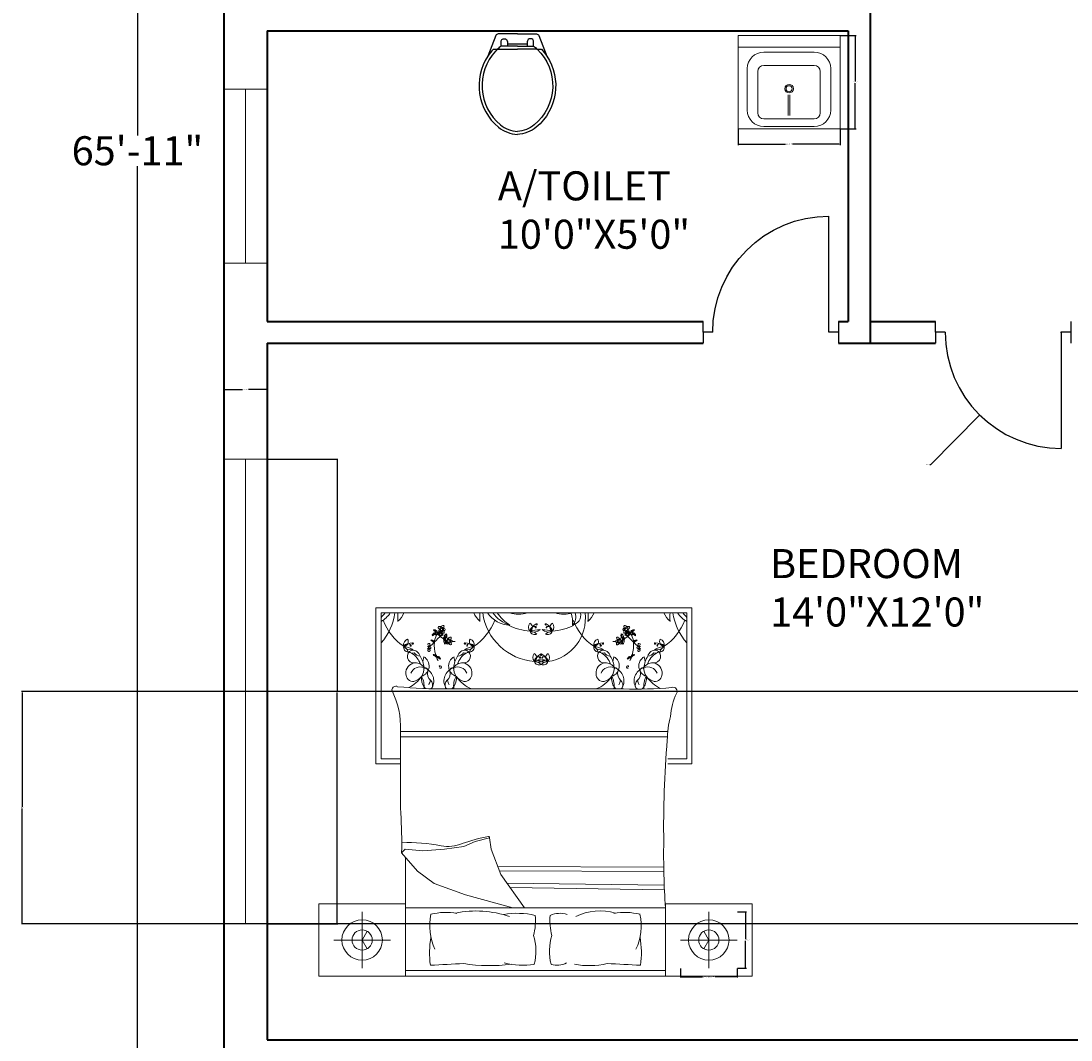
# Model space of a CAD drawing. Units: inches. Extents: x -19 to 419, y -828 to 43.
# Tile 6 of 9: x -19 to 198, y -574 to -364. Entities that reach past the tile are written whole.
import ezdxf

# ---------------------------------------------------------------- set-up
doc = ezdxf.new("R2010")
doc.units = ezdxf.units.IN
doc.header["$MEASUREMENT"] = 0
for name, color, linetype, lineweight in [('A-ANNO-DIMS', 2, 'Continuous', 18), ('A-AREA-IDEN', 7, 'Continuous', 25), ('A-DOOR', 3, 'Continuous', 25), ('A-FLOR-FIXT', 9, 'Continuous', 20), ('A-FURN', 8, 'Continuous', 18), ('A-GLAZ', 4, 'Continuous', 20), ('A-WALL', 7, 'Continuous', 40)]:
    doc.layers.add(name, color=color, linetype=linetype, lineweight=lineweight)
doc.layers.add('WC-Detail_dwgmodels.com', color=251, linetype='Continuous')
doc.layers.add('WC-Outline_dwgmodels.com', color=250, linetype='Continuous')
doc.styles.get("Standard").update_dxf_attribs({"font": 'arial.ttf'})
doc.dimstyles.get("Standard").update_dxf_attribs({"dimtxt": 0.18, "dimasz": 0.18, "dimexe": 0.18, "dimexo": 0.0625, "dimgap": 0.09, "dimtad": 0, "dimtih": 1, "dimtoh": 1, "dimdec": 0, "dimzin": 0, "dimdsep": 46, "dimlunit": 3, "dimtxsty": 'Standard', "dimcen": 0.09, "dimadec": 0, "dimazin": 0, "dimtfac": 1, "dimtdec": 0, "dimtofl": 0, "dimtmove": 0, "dimatfit": 3, "dimfxl": 1, "dimtolj": 1, "dimtzin": 0, "dimarcsym": 0})

# ---------------------------------------------------------------- blocks, each defined once
blk = doc.blocks.new('*D2')
at = {"layer": 'A-ANNO-DIMS', "color": 0, "lineweight": -2, "transparency": 16777216}
for p, q in [((22.68, 4.77), (4.74, 4.77)), ((4.92, 4.59), (4.92, -387.33)), ((4.92, -785.55), (4.92, -393.64)), ((22.68, -785.73), (4.74, -785.73))]:
    blk.add_line(p, q, dxfattribs=at)
at = {"layer": 'A-ANNO-DIMS', "color": 0, "transparency": 16777216}
for points in [[(4.89, 4.59), (4.95, 4.59), (4.92, 4.77)], [(4.89, -785.55), (4.95, -785.55), (4.92, -785.73)]]:
    blk.add_solid(points, dxfattribs=at)
at = {"layer": 'Defpoints', "color": 0, "transparency": 16777216}
for p in [(22.74, 4.77), (4.92, -785.73), (22.74, -785.73)]:
    blk.add_point(p, dxfattribs=at)
at = {"layer": 'A-ANNO-DIMS', "color": 0, "transparency": 16777216, "insert": (4.92, -390.48), "char_height": 6, "attachment_point": 5}
blk.add_mtext('\\A1;65\'-11"', dxfattribs=at)
blk = doc.blocks.new('М14 600х655')
for p, q in [((-655, 600), (-655, 0)), ((-655, 600), (-655, 0)), ((-655, 0), (-655, 600)), ((0, 600), (-655, 600)), ((0, 0), (0, 600)), ((0, 525), (-655, 525)), ((-165.1, 494.1), (-489.9, 494.1)), ((-165.4, 408.4), (-490.2, 408.4)), ((-595.8, 388.1), (-595.8, 121.3)), ((-528.4, 370.1), (-528.4, 103.3)), ((-127.2, 103.3), (-127.2, 370.1)), ((-59.2, 121.3), (-59.2, 388.1)), ((-333.5, 87.1), (-333.5, 219.6)), ((-321.5, 87.1), (-321.5, 219.6)), ((-655, 0), (-655, 0)), ((-655, 0), (-655, 0)), ((-655, 0), (0, 0)), ((-655, 0), (0, 0)), ((-490.2, 65.1), (-165.4, 65.1)), ((-489.9, 15.4), (-165.1, 15.4))]:
    blk.add_line(p, q)
for radius in [27.6, 19.3]:
    blk.add_circle((-327.5, 258.9), radius)
for centre, radius, start, end in [((-489.9, 388.1), 105.9, 90, 180), ((-165.1, 388.1), 105.9, 0, 90), ((-490.2, 370.1), 38.2, 90, 180), ((-165.4, 370.1), 38.2, 0, 90), ((-489.9, 121.3), 105.9, 180, 270), ((-490.2, 103.3), 38.2, 180, 270), ((-165.4, 103.3), 38.2, 270, 0), ((-165.1, 121.3), 105.9, 270, 0)]:
    blk.add_arc(centre, radius, start, end)
blk = doc.blocks.new('WIN-36X9')
for p, q in [((36, 9), (0, 9)), ((0, 9), (0, 0)), ((36, 0), (36, 9)), ((0, 4.5), (36, 4.5)), ((0, 0), (36, 0))]:
    blk.add_line(p, q)
blk = doc.blocks.new('WIN-96X9')
for p, q in [((96, 9), (0, 9)), ((0, 9), (0, 0)), ((96, 0), (96, 9)), ((0, 4.5), (96, 4.5)), ((0, 0), (96, 0))]:
    blk.add_line(p, q)
blk = doc.blocks.new('DOOR-24-PARTITION')
for p, q in [((2, 2.25), (2, 26.25)), ((0, 4.5), (0, 0)), ((28, 2.25), (28, 4.5)), ((0, 2.25), (2, 2.25)), ((26, 2.25), (28, 2.25)), ((28, 2.25), (28, 0))]:
    blk.add_line(p, q)
blk.add_arc((2, 2.25), 24, 0, 90)
blk = doc.blocks.new('BEDSIDE-LAMP')
for p, q in [((5.85, 11.69), (5.85, 0)), ((0, 5.85), (11.69, 5.85))]:
    blk.add_line(p, q)
for points in [[(5.85, 5.85), (4.8, 7.66)], [(5.85, 5.85), (4.8, 4.04)]]:
    blk.add_lwpolyline(points)
for radius in [4.18, 2.09]:
    blk.add_circle((5.85, 5.85), radius)
blk = doc.blocks.new('*D20')
at = {"layer": 'A-ANNO-DIMS', "color": 0, "lineweight": -2, "transparency": 16777216}
for p, q in [((31.8, -454.23), (46.32, -454.23)), ((46.14, -454.41), (46.14, -502.05)), ((46.14, -550.05), (46.14, -502.42)), ((31.8, -550.23), (46.32, -550.23))]:
    blk.add_line(p, q, dxfattribs=at)
at = {"layer": 'A-ANNO-DIMS', "color": 0, "transparency": 16777216}
for points in [[(46.11, -454.41), (46.17, -454.41), (46.14, -454.23)], [(46.11, -550.05), (46.17, -550.05), (46.14, -550.23)]]:
    blk.add_solid(points, dxfattribs=at)
at = {"layer": 'Defpoints', "color": 0, "transparency": 16777216}
for p in [(31.74, -454.23), (31.74, -550.23), (46.14, -550.23)]:
    blk.add_point(p, dxfattribs=at)
at = {"layer": 'A-ANNO-DIMS', "color": 0, "transparency": 16777216, "insert": (46.14, -502.23), "char_height": 0.18, "attachment_point": 5}
blk.add_mtext('\\A1;W3 8\'-0" TYP.', dxfattribs=at)
blk = doc.blocks.new('*D21')
at = {"layer": 'A-ANNO-DIMS', "color": 0, "lineweight": -2, "transparency": 16777216}
for p, q in [((22.74, -454.17), (22.74, -439.65)), ((22.92, -439.83), (26.6, -439.83)), ((31.56, -439.83), (27.88, -439.83)), ((31.74, -454.17), (31.74, -439.65))]:
    blk.add_line(p, q, dxfattribs=at)
at = {"layer": 'A-ANNO-DIMS', "color": 0, "transparency": 16777216}
for points in [[(22.92, -439.8), (22.92, -439.86), (22.74, -439.83)], [(31.56, -439.8), (31.56, -439.86), (31.74, -439.83)]]:
    blk.add_solid(points, dxfattribs=at)
at = {"layer": 'Defpoints', "color": 0, "transparency": 16777216}
for p in [(31.74, -439.83), (22.74, -454.23), (31.74, -454.23)]:
    blk.add_point(p, dxfattribs=at)
at = {"layer": 'A-ANNO-DIMS', "color": 0, "transparency": 16777216, "insert": (27.24, -439.83), "char_height": 0.18, "attachment_point": 5}
blk.add_mtext('\\A1;0\'-9" TYP.', dxfattribs=at)
blk = doc.blocks.new('*D30')
at = {"layer": 'A-ANNO-DIMS', "color": 0, "lineweight": -2, "transparency": 16777216}
for p, q in [((128.98, -386.03), (128.98, -389.31)), ((150.03, -386.03), (150.03, -389.31)), ((129.16, -389.13), (138.77, -389.13)), ((149.85, -389.13), (140.24, -389.13))]:
    blk.add_line(p, q, dxfattribs=at)
at = {"layer": 'A-ANNO-DIMS', "color": 0, "transparency": 16777216}
for points in [[(129.16, -389.1), (129.16, -389.16), (128.98, -389.13)], [(149.85, -389.1), (149.85, -389.16), (150.03, -389.13)]]:
    blk.add_solid(points, dxfattribs=at)
at = {"layer": 'Defpoints', "color": 0, "transparency": 16777216}
for p in [(128.98, -385.97), (150.03, -385.97), (150.03, -389.13)]:
    blk.add_point(p, dxfattribs=at)
at = {"layer": 'A-ANNO-DIMS', "color": 0, "transparency": 16777216, "insert": (139.5, -389.13), "char_height": 0.18, "attachment_point": 5}
blk.add_mtext('\\A1;BASIN 1\'-9"', dxfattribs=at)
blk = doc.blocks.new('*D31')
at = {"layer": 'A-ANNO-DIMS', "color": 0, "lineweight": -2, "transparency": 16777216}
for p, q in [((150.09, -366.69), (153.37, -366.69)), ((153.19, -366.87), (153.19, -376.15)), ((153.19, -385.79), (153.19, -376.51)), ((150.09, -385.97), (153.37, -385.97))]:
    blk.add_line(p, q, dxfattribs=at)
at = {"layer": 'A-ANNO-DIMS', "color": 0, "transparency": 16777216}
for points in [[(153.16, -366.87), (153.22, -366.87), (153.19, -366.69)], [(153.16, -385.79), (153.22, -385.79), (153.19, -385.97)]]:
    blk.add_solid(points, dxfattribs=at)
at = {"layer": 'Defpoints', "color": 0, "transparency": 16777216}
for p in [(150.03, -366.69), (153.19, -366.69), (150.03, -385.97)]:
    blk.add_point(p, dxfattribs=at)
at = {"layer": 'A-ANNO-DIMS', "color": 0, "transparency": 16777216, "insert": (153.19, -376.33), "char_height": 0.18, "attachment_point": 5}
blk.add_mtext('\\A1;1\'-7 1/2"', dxfattribs=at)
blk = doc.blocks.new('*D38')
at = {"layer": 'A-ANNO-DIMS', "color": 0, "lineweight": -2, "transparency": 16777216}
for p, q in [((117.08, -559.48), (117.08, -561.35)), ((128.77, -559.48), (128.77, -561.35)), ((117.26, -561.17), (121.63, -561.17)), ((128.59, -561.17), (124.22, -561.17))]:
    blk.add_line(p, q, dxfattribs=at)
at = {"layer": 'A-ANNO-DIMS', "color": 0, "transparency": 16777216}
for points in [[(117.26, -561.14), (117.26, -561.2), (117.08, -561.17)], [(128.59, -561.14), (128.59, -561.2), (128.77, -561.17)]]:
    blk.add_solid(points, dxfattribs=at)
at = {"layer": 'Defpoints', "color": 0, "transparency": 16777216}
for p in [(117.08, -559.42), (128.77, -559.42), (128.77, -561.17)]:
    blk.add_point(p, dxfattribs=at)
at = {"layer": 'A-ANNO-DIMS', "color": 0, "transparency": 16777216, "insert": (122.93, -561.17), "char_height": 0.18, "attachment_point": 5}
blk.add_mtext('\\A1;LAMP 0\'-11 1/2" TYP.', dxfattribs=at)
blk = doc.blocks.new('*D39')
at = {"layer": 'A-ANNO-DIMS', "color": 0, "lineweight": -2, "transparency": 16777216}
for p, q in [((128.84, -547.72), (130.71, -547.72)), ((130.53, -547.9), (130.53, -553.39)), ((130.53, -559.24), (130.53, -553.75)), ((128.84, -559.42), (130.71, -559.42))]:
    blk.add_line(p, q, dxfattribs=at)
at = {"layer": 'A-ANNO-DIMS', "color": 0, "transparency": 16777216}
for points in [[(130.5, -547.9), (130.56, -547.9), (130.53, -547.72)], [(130.5, -559.24), (130.56, -559.24), (130.53, -559.42)]]:
    blk.add_solid(points, dxfattribs=at)
at = {"layer": 'Defpoints', "color": 0, "transparency": 16777216}
for p in [(128.77, -547.72), (130.53, -547.72), (128.77, -559.42)]:
    blk.add_point(p, dxfattribs=at)
at = {"layer": 'A-ANNO-DIMS', "color": 0, "transparency": 16777216, "insert": (130.53, -553.57), "char_height": 0.18, "attachment_point": 5}
blk.add_mtext('\\A1;0\'-11 1/2" TYP.', dxfattribs=at)
blk = doc.blocks.new('*D44')
at = {"layer": 'A-ANNO-DIMS', "color": 0, "lineweight": -2, "transparency": 16777216}
for p, q in [((258.18, -502.23), (-19.04, -502.23)), ((-18.86, -502.41), (-18.86, -526.05)), ((-18.86, -550.05), (-18.86, -526.42)), ((258.18, -550.23), (-19.04, -550.23))]:
    blk.add_line(p, q, dxfattribs=at)
at = {"layer": 'A-ANNO-DIMS', "color": 0, "transparency": 16777216}
for points in [[(-18.89, -502.41), (-18.83, -502.41), (-18.86, -502.23)], [(-18.89, -550.05), (-18.83, -550.05), (-18.86, -550.23)]]:
    blk.add_solid(points, dxfattribs=at)
at = {"layer": 'Defpoints', "color": 0, "transparency": 16777216}
for p in [(-18.86, -502.23), (258.24, -502.23), (258.24, -550.23)]:
    blk.add_point(p, dxfattribs=at)
at = {"layer": 'A-ANNO-DIMS', "color": 0, "transparency": 16777216, "insert": (-18.86, -526.23), "char_height": 0.18, "attachment_point": 5}
blk.add_mtext('\\A1;4\'-0"', dxfattribs=at)
blk = doc.blocks.new('*D50')
at = {"layer": 'A-ANNO-DIMS', "color": 0, "lineweight": -2, "transparency": 16777216}
for p, q in [((195.65, -427.98), (195.83, -427.98)), ((195.74, -428.07), (195.74, -427.89)), ((168.78, -455.33), (178.77, -445.2)), ((168.6, -455.33), (168.78, -455.33))]:
    blk.add_line(p, q, dxfattribs=at)
at = {"layer": 'A-ANNO-DIMS', "color": 0, "transparency": 16777216}
blk.add_solid([(178.74, -445.18), (178.79, -445.23), (178.89, -445.08)], dxfattribs=at)
at = {"layer": 'Defpoints', "color": 0, "transparency": 16777216}
for p in [(195.74, -427.98), (178.89, -445.08)]:
    blk.add_point(p, dxfattribs=at)
at = {"layer": 'A-ANNO-DIMS', "color": 0, "transparency": 16777216, "insert": (168.19, -455.33), "char_height": 0.18, "attachment_point": 5}
blk.add_mtext('\\A1;R2\'-0"', dxfattribs=at)

msp = doc.modelspace()

# ---------------------------------------------------------------- linework, layer by layer
at = {"layer": 'A-FURN'}
for p, q in [((54.19, -484.92), (54.19, -517.16)), ((119.44, -484.92), (54.19, -484.92)), ((119.44, -517.16), (119.44, -484.92)), ((55.23, -485.96), (118.4, -485.96)), ((55.23, -516.12), (55.23, -485.96)), ((118.4, -485.96), (118.4, -516.12)), ((64.05, -495.03), (63.85, -496.04)), ((70.3, -495.03), (70.5, -496.04)), ((103.33, -495.03), (103.13, -496.04)), ((109.58, -495.03), (109.78, -496.04)), ((105.3, -501.67), (68.96, -501.67)), ((114.47, -510.46), (59.25, -510.46)), ((114.38, -511.58), (59.25, -511.58)), ((59.25, -516.12), (55.23, -516.12)), ((118.4, -516.12), (114.46, -516.12)), ((54.19, -517.16), (59.25, -517.16)), ((114.48, -517.16), (119.44, -517.16)), ((74.7, -533.18), (72.35, -534.26)), ((77.6, -532.45), (74.7, -533.18)), ((77.97, -534.81), (77.6, -532.45)), ((60.2, -534.81), (59.48, -535.53)), ((59.48, -535.53), (62.74, -539.34)), ((63.83, -535.17), (60.2, -534.81)), ((68.36, -534.81), (63.83, -535.17)), ((72.35, -534.26), (68.36, -534.81)), ((79.96, -540.06), (77.97, -534.81)), ((60.28, -561.03), (60.28, -536.47)), ((62.74, -539.34), (66.18, -541.87)), ((113.66, -538.51), (79.32, -538.37)), ((113.66, -539.43), (79.67, -539.3)), ((66.18, -541.87), (72.71, -544.23)), ((84.86, -546.89), (79.96, -540.06)), ((113.7, -542.25), (81.2, -541.79)), ((72.71, -544.23), (82.47, -546.89)), ((113.74, -543.17), (81.87, -542.72)), ((60.28, -546.89), (113.98, -546.89)), ((42.38, -561.03), (131.88, -561.03)), ((113.98, -559.88), (60.28, -559.88))]:
    msp.add_line(p, q, dxfattribs=at)
for points in [[(59.29, -527.34, -0.001242), (59.25, -510.36, 0.127202), (57.45, -501.89)], [(114.36, -512.28, -0.056112), (115.01, -507.36, -0.095341), (116.27, -502.61)], [(65.42, -558.8, -0.074897), (65.53, -552.95, 0.472817)], [(86.71, -552.63, -0.14099), (86.89, -558.59, -0.235245)], [(90.53, -552.63, 0.14099), (90.35, -558.59, 0.235245)], [(108.84, -558.8, 0.074897), (108.73, -552.95, -0.472817)]]:
    msp.add_lwpolyline(points, format="xyb", dxfattribs=at)
for points in [[(60.28, -546.11), (42.38, -546.11), (42.38, -561.03)], [(113.98, -561.03), (113.98, -546.11), (131.88, -546.11), (131.88, -561.03)]]:
    msp.add_lwpolyline(points, dxfattribs=at)
for centre in [(67.73, -489.38), (105.9, -489.38), (69.22, -491.79), (104.41, -491.79)]:
    msp.add_circle(centre, 0.228, dxfattribs=at)
for centre, radius, start, end in [((50.34, -481.75), 7.1, 313.5186, 323.6964), ((52.39, -482.82), 5.69, 299.8884, 326.5383), ((46.53, -484.38), 11.69, 318.1144, 352.255), ((66.52, -483.23), 11.69, 201.4092, 235.6135), ((55.58, -484.13), 4.75, 311.0454, 337.4453), ((42.56, -486.69), 16.17, 356.3481, 2.5919), ((78.77, -484.13), 4.75, 202.5547, 228.9546), ((67.83, -483.23), 11.69, 304.3865, 338.5908), ((91.79, -486.69), 16.17, 177.4081, 183.6519), ((87.82, -484.38), 11.69, 187.745, 265.5377), ((81.96, -482.82), 5.69, 213.4617, 268.728), ((84.01, -481.75), 7.1, 216.3036, 252.1496), ((87.74, -479.76), 10.56, 215.947, 235.9877), ((83.66, -479.81), 6.43, 252.9798, 286.4569), ((86.21, -476.5), 9.5, 264.3643, 265.6213), ((91.21, -469.99), 16.98, 250.0972, 250.2783), ((88.41, -487.08), 9.04, 278.1803, 7.1364), ((92.95, -479.81), 6.43, 253.5431, 287.0202), ((90.41, -476.5), 9.5, 274.3787, 275.6357), ((85.4, -469.99), 16.98, 289.7217, 289.9028), ((89.58, -487.91), 5.23, 353.3805, 21.883), ((94.38, -486.45), 2.1, 280.9261, 13.6102), ((92.81, -486.74), 2.65, 318.0951, 17.1391), ((105.8, -483.23), 11.69, 201.4092, 235.6135), ((81.84, -486.69), 16.17, 356.3481, 2.5919), ((94.86, -484.13), 4.75, 311.0454, 337.4453), ((118.05, -484.13), 4.75, 202.5547, 228.9546), ((107.11, -483.23), 11.69, 304.3865, 338.5908), ((131.07, -486.69), 16.17, 177.4081, 183.6519), ((127.1, -484.38), 11.69, 187.745, 221.8856), ((121.24, -482.82), 5.69, 213.4617, 240.1116), ((123.29, -481.75), 7.1, 216.3036, 226.4814), ((66.43, -490.66), 0.593, 82.6008, 147.1845), ((66.26, -489.72), 0.254, 55.6077, 145.6462), ((66.08, -490.26), 0.689, 21.7087, 93.0299), ((62.45, -495.18), 6.66, 53.6254, 57.3216), ((66.3, -490.09), 0.593, 342.8042, 79.6943), ((66.25, -490.03), 0.263, 338.2452, 53.6254), ((66.67, -490.2), 0.199, 158.2452, 340.6395), ((70.41, -488.54), 3.97, 201.7087, 206.2181), ((69.94, -492.36), 3.72, 137.5083, 145.9967), ((67.36, -490.66), 0.631, 61.1838, 141.6792), ((67.25, -488.96), 0.226, 134.3732, 211.9501), ((67.67, -488.7), 0.719, 211.9501, 255.2442), ((67.26, -489.21), 0.45, 8.5614, 112.5914), ((67.48, -489.7), 0.311, 88.5719, 233.8954), ((67.44, -489.79), 0.223, 228.2946, 6.2474), ((67.39, -489.19), 0.151, 352.868, 97.094), ((67.23, -489.52), 0.314, 298.8493, 359.9355), ((67.31, -489.79), 0.358, 4.2123, 48.1587), ((68.04, -488.96), 0.376, 100.9597, 208.7804), ((68.04, -489.74), 0.38, 183.635, 258.4363), ((67.31, -490.77), 0.755, 15.6484, 62.2957), ((67.99, -489.6), 0.218, 178.1325, 268.8919), ((68.44, -489.46), 0.692, 132.3896, 156.5724), ((68.14, -489.55), 0.373, 42.3208, 130.2111), ((68.22, -489.16), 0.471, 226.3462, 279.6513), ((67.74, -490.03), 0.548, 7.4968, 71.2737), ((67.72, -488.76), 0.53, 291.6382, 4.947), ((68.14, -488.67), 0.746, 254.2829, 276.9148), ((68.07, -488.73), 0.175, 4.947, 127.5263), ((68.11, -490.01), 0.176, 215.0752, 14.7644), ((68.27, -489.43), 0.196, 279.6513, 42.3208), ((86.93, -478.12), 11.69, 242.5854, 265.5377), ((86.98, -488.9), 1.3, 140.8855, 222.2127), ((85.51, -488.94), 0.976, 301.6373, 61.4609), ((88.82, -490.73), 2.96, 121.989, 161.0841), ((86.97, -489.74), 0.956, 76.148, 182.2415), ((88.46, -497.57), 8.18, 92.7418, 107.407), ((86.78, -488.09), 1.85, 245.6899, 314.4589), ((85.97, -491.77), 2, 44.6273, 88.5415), ((86.95, -489.5), 0.969, 196.1963, 296.9726), ((87.17, -488.93), 0.126, 140.0755, 76.148), ((87.33, -488.35), 0.145, 288.4408, 121.989), ((87.35, -488.42), 0.0705, 171.9833, 288.4408), ((88.15, -497.57), 8.18, 72.593, 87.2582), ((89.83, -488.09), 1.85, 225.5411, 294.3101), ((89.29, -488.35), 0.145, 58.011, 251.5592), ((90.65, -491.77), 2, 91.4585, 135.3727), ((89.66, -489.5), 0.969, 243.0274, 343.8037), ((89.26, -488.42), 0.0705, 251.5592, 8.0167), ((89.43, -488.98), 0.0762, 103.9791, 39.8091), ((87.8, -490.73), 2.96, 18.9159, 58.011), ((89.64, -489.74), 0.956, 357.7585, 103.852), ((91.11, -488.94), 0.976, 118.5391, 238.3627), ((89.63, -488.9), 1.3, 317.7873, 39.1145), ((89.69, -478.12), 11.69, 274.4623, 297.4146), ((105.36, -489.43), 0.196, 137.6792, 260.3487), ((105.49, -489.55), 0.373, 49.7889, 137.6792), ((105.41, -489.16), 0.471, 260.3487, 313.6538), ((105.52, -490.01), 0.176, 165.2356, 324.9248), ((105.89, -490.03), 0.548, 108.7263, 172.5032), ((105.56, -488.73), 0.175, 52.4737, 175.053), ((105.91, -488.76), 0.53, 175.053, 248.3618), ((105.49, -488.67), 0.746, 263.0852, 285.7171), ((106.32, -490.77), 0.755, 117.7043, 164.3516), ((105.64, -489.6), 0.218, 271.1081, 1.8675), ((105.19, -489.46), 0.692, 23.4276, 47.6104), ((105.59, -488.96), 0.376, 331.2196, 79.0403), ((105.59, -489.74), 0.38, 281.5637, 356.365), ((106.37, -489.21), 0.45, 67.4086, 171.4386), ((106.32, -489.79), 0.358, 131.8413, 175.7877), ((106.19, -489.79), 0.223, 173.7526, 311.7054), ((106.27, -490.66), 0.631, 38.3208, 118.8162), ((106.4, -489.52), 0.314, 180.0645, 241.1507), ((106.24, -489.19), 0.151, 82.906, 187.132), ((105.96, -488.7), 0.719, 284.7558, 328.0499), ((106.15, -489.7), 0.311, 306.1046, 91.4281), ((103.69, -492.36), 3.72, 34.0033, 42.4917), ((106.38, -488.96), 0.226, 328.0499, 45.6268), ((107.33, -490.09), 0.593, 100.3057, 197.1958), ((106.96, -490.2), 0.199, 199.3605, 21.7548), ((103.22, -488.54), 3.97, 333.7819, 338.2913), ((107.55, -490.26), 0.689, 86.9701, 158.2913), ((107.38, -490.03), 0.263, 126.3746, 201.7548), ((107.2, -490.66), 0.593, 32.8155, 97.3992), ((107.37, -489.72), 0.254, 34.3538, 124.3923), ((111.18, -495.18), 6.66, 122.6784, 126.3746), ((61.19, -492.59), 1.3, 110.9613, 192.2885), ((59.89, -491.89), 0.976, 271.7131, 31.5367), ((61.87, -495.1), 2.96, 92.0648, 131.1598), ((61.77, -492.29), 0.145, 258.5166, 92.0648), ((60.04, -486.24), 8.5, 307.9541, 316.8459), ((65.56, -494.1), 2.52, 82.8698, 91.6736), ((65.91, -491.37), 0.47, 205.5379, 258.6744), ((65.24, -492.97), 1.41, 59.344, 79.7412), ((66.07, -490.55), 0.254, 123.0979, 213.1364), ((64.93, -492.96), 1.44, 43.6929, 51.7899), ((66.51, -490.92), 0.689, 92.3172, 160.5201), ((69.66, -496.15), 6.66, 121.1156, 124.8118), ((65.81, -492.02), 0.43, 355.7131, 81.6568), ((65.57, -492.4), 0.75, 27.3659, 59.344), ((66.14, -491.9), 0.182, 202.5583, 304.2343), ((66.35, -490.68), 0.263, 45.7354, 121.1156), ((73.64, -492.55), 7.41, 176.1723, 196.4158), ((69.94, -492.36), 3.72, 150.7959, 175.244), ((75.29, -500.27), 12.23, 127.8256, 137.7588), ((66.68, -490.35), 0.199, 225.7354, 48.1297), ((67.25, -491.25), 1.04, 40.9365, 112.7695), ((66.91, -490.9), 0.611, 49.3812, 95.5456), ((70.33, -487.42), 4.46, 220.182, 239.456), ((67.79, -489.88), 0.735, 229.3812, 289.9959), ((67.74, -490.28), 1.04, 287.889, 359.722), ((67.71, -490.77), 0.611, 305.1128, 351.2773), ((68.03, -491.89), 0.631, 3.8774, 87.1501), ((67.58, -491.65), 0.611, 352.0748, 38.2393), ((67.47, -492.13), 1.04, 343.6301, 55.4631), ((68.92, -491.83), 0.735, 172.0748, 232.6895), ((68.21, -490.66), 0.631, 271.4625, 339.4747), ((69.04, -490.97), 0.735, 110.6625, 171.2773), ((67.91, -491.92), 0.755, 318.342, 4.9894), ((68.74, -491.36), 0.226, 134.3732, 211.9501), ((70.33, -487.42), 4.46, 246.1523, 246.9499), ((69.16, -491.1), 0.719, 211.9501, 255.2442), ((68.75, -491.61), 0.45, 8.5614, 112.5914), ((68.97, -492.1), 0.311, 88.5719, 233.8954), ((68.1, -490.6), 0.755, 338.3627, 25.0101), ((68.93, -492.19), 0.223, 228.2946, 6.2474), ((68.88, -491.59), 0.151, 352.868, 97.094), ((68.72, -491.92), 0.314, 298.8493, 359.9355), ((68.8, -492.19), 0.358, 4.2123, 48.1587), ((69.53, -491.36), 0.376, 100.9597, 208.7804), ((69.53, -492.14), 0.38, 183.635, 258.4363), ((69.48, -492), 0.218, 178.1325, 268.8919), ((69.94, -491.87), 0.692, 132.3896, 156.5724), ((69.63, -491.95), 0.373, 42.3208, 130.2111), ((69.72, -491.56), 0.471, 226.3462, 279.6513), ((69.23, -492.44), 0.548, 7.4968, 71.2737), ((69.21, -491.16), 0.53, 291.6382, 4.947), ((69.63, -491.07), 0.746, 254.2829, 276.9148), ((69.56, -491.13), 0.175, 4.947, 127.5263), ((69.76, -491.84), 0.196, 279.6513, 42.3208), ((70.33, -487.42), 4.46, 265.2415, 272.8929), ((72.58, -492.29), 0.145, 87.9352, 281.4834), ((72.48, -495.1), 2.96, 48.8402, 87.9352), ((74.46, -491.89), 0.976, 148.4633, 268.2869), ((73.16, -492.59), 1.3, 347.7115, 69.0387), ((100.47, -492.59), 1.3, 110.9613, 192.2885), ((99.17, -491.89), 0.976, 271.7131, 31.5367), ((101.15, -495.1), 2.96, 92.0648, 131.1598), ((101.05, -492.29), 0.145, 258.5166, 92.0648), ((103.3, -487.42), 4.46, 267.1071, 274.7585), ((103.87, -491.84), 0.196, 137.6792, 260.3487), ((104, -491.95), 0.373, 49.7889, 137.6792), ((103.91, -491.56), 0.471, 260.3487, 313.6538), ((104.4, -492.44), 0.548, 108.7263, 172.5032), ((104.07, -491.13), 0.175, 52.4737, 175.053), ((104.42, -491.16), 0.53, 175.053, 248.3618), ((104, -491.07), 0.746, 263.0852, 285.7171), ((104.15, -492), 0.218, 271.1081, 1.8675), ((103.69, -491.87), 0.692, 23.4276, 47.6104), ((104.1, -491.36), 0.376, 331.2196, 79.0403), ((104.1, -492.14), 0.38, 281.5637, 356.365), ((104.88, -491.61), 0.45, 67.4086, 171.4386), ((104.7, -492.19), 0.223, 173.7526, 311.7054), ((104.83, -492.19), 0.358, 131.8413, 175.7877), ((104.91, -491.92), 0.314, 180.0645, 241.1507), ((104.75, -491.59), 0.151, 82.906, 187.132), ((104.47, -491.1), 0.719, 284.7558, 328.0499), ((104.66, -492.1), 0.311, 306.1046, 91.4281), ((105.53, -490.6), 0.755, 154.9899, 201.6373), ((105.42, -490.66), 0.631, 200.5253, 268.5375), ((105.89, -490.28), 1.04, 180.278, 252.111), ((104.59, -490.97), 0.735, 8.7227, 69.3375), ((105.6, -491.89), 0.631, 92.8499, 176.1226), ((105.72, -491.92), 0.755, 175.0106, 221.658), ((104.89, -491.36), 0.226, 328.0499, 45.6268), ((103.3, -487.42), 4.46, 293.0501, 293.8477), ((106.16, -492.13), 1.04, 124.5369, 196.3699), ((104.71, -491.83), 0.735, 307.3105, 7.9252), ((105.92, -490.77), 0.611, 188.7227, 234.8872), ((106.05, -491.65), 0.611, 141.7607, 187.9252), ((103.3, -487.42), 4.46, 300.544, 319.818), ((106.38, -491.25), 1.04, 67.2305, 139.0635), ((105.84, -489.88), 0.735, 250.0041, 310.6188), ((98.34, -500.27), 12.23, 42.2412, 52.1744), ((106.72, -490.9), 0.611, 84.4544, 130.6188), ((106.95, -490.35), 0.199, 131.8703, 314.2646), ((103.69, -492.36), 3.72, 4.756, 29.2041), ((107.28, -490.68), 0.263, 58.8844, 134.2646), ((99.99, -492.55), 7.41, 343.5842, 3.8277), ((107.12, -490.92), 0.689, 19.4799, 87.6828), ((107.82, -492.02), 0.43, 98.3432, 184.2869), ((108.06, -492.4), 0.75, 120.656, 152.6341), ((107.49, -491.9), 0.182, 235.7657, 337.4417), ((113.59, -486.24), 8.5, 223.1541, 232.0459), ((103.97, -496.15), 6.66, 55.1882, 58.8844), ((108.7, -492.96), 1.44, 128.2101, 136.3071), ((108.4, -492.97), 1.41, 100.2588, 120.656), ((107.56, -490.55), 0.254, 326.8636, 56.9021), ((108.07, -494.1), 2.52, 88.3264, 97.1302), ((107.72, -491.37), 0.47, 281.3256, 334.4621), ((111.86, -492.29), 0.145, 87.9352, 281.4834), ((111.76, -495.1), 2.96, 48.8402, 87.9352), ((113.74, -491.89), 0.976, 148.4633, 268.2869), ((112.44, -492.59), 1.3, 347.7115, 69.0387), ((60.86, -493.1), 0.969, 166.272, 267.0484), ((60.77, -493.31), 0.956, 46.2238, 152.3173), ((58.15, -500.85), 8.18, 62.8176, 77.4827), ((61.42, -491.79), 1.85, 215.7657, 284.5347), ((58.88, -494.57), 2, 14.7031, 58.6173), ((62, -494.96), 1.34, 109.1312, 279.736), ((61.72, -493.5), 0.823, 216.7319, 296.0245), ((61.34, -492.72), 0.126, 110.2817, 46.2238), ((59.34, -497.91), 4.23, 18.2955, 58.7386), ((61.68, -495.36), 1.68, 15.6955, 94.031), ((61.75, -492.36), 0.0705, 142.0591, 258.5166), ((63.49, -493.13), 1.79, 218.4175, 263.8338), ((65.11, -492.72), 0.376, 100.9597, 142.2379), ((64.8, -493.14), 0.228, 273.2768, 86.7232), ((65.12, -493.49), 0.38, 217.3642, 258.4363), ((65.07, -493.36), 0.218, 178.1325, 268.8919), ((65.52, -493.22), 0.692, 132.3896, 156.5724), ((65.21, -493.31), 0.373, 42.3208, 130.2111), ((65.3, -492.92), 0.471, 226.3462, 279.6513), ((64.79, -492.52), 0.53, 291.6382, 4.947), ((64.81, -493.79), 0.548, 7.4968, 71.2737), ((65.21, -492.43), 0.746, 254.2829, 276.9148), ((65.15, -492.49), 0.175, 4.947, 127.5263), ((65.18, -493.77), 0.176, 215.0752, 14.7644), ((65.34, -493.19), 0.196, 279.6513, 42.3208), ((69.6, -492.41), 0.176, 215.0752, 14.7644), ((75.01, -497.91), 4.23, 121.2614, 161.7045), ((72.67, -495.36), 1.68, 85.969, 164.3045), ((70.87, -493.13), 1.79, 276.1662, 321.5825), ((72.35, -494.96), 1.34, 260.264, 70.8688), ((72.63, -493.5), 0.823, 243.9755, 323.2681), ((72.93, -491.79), 1.85, 255.4653, 324.2343), ((76.2, -500.85), 8.18, 102.5173, 117.1824), ((72.6, -492.36), 0.0705, 281.4834, 37.9409), ((73.58, -493.31), 0.956, 27.6827, 133.7762), ((73.02, -492.76), 0.0762, 133.7729, 69.7333), ((73.49, -493.1), 0.969, 272.9516, 13.728), ((75.47, -494.57), 2, 121.3827, 165.2969), ((87.87, -495.16), 1.3, 140.8855, 222.2127), ((86.4, -495.2), 0.976, 301.6373, 61.4609), ((88.22, -494.61), 0.145, 288.4408, 121.989), ((88.39, -494.61), 0.145, 58.011, 251.5592), ((90.21, -495.2), 0.976, 118.5391, 238.3627), ((88.74, -495.16), 1.3, 317.7873, 39.1145), ((100.14, -493.1), 0.969, 166.272, 267.0484), ((100.05, -493.31), 0.956, 46.2238, 152.3173), ((98.16, -494.57), 2, 14.7031, 58.6173), ((100.7, -491.79), 1.85, 215.7657, 284.5347), ((97.43, -500.85), 8.18, 62.8176, 77.4827), ((101.28, -494.96), 1.34, 109.1312, 279.736), ((101, -493.5), 0.823, 216.7319, 296.0245), ((100.62, -492.72), 0.126, 110.2817, 46.2238), ((98.62, -497.91), 4.23, 18.2955, 58.7386), ((100.96, -495.36), 1.68, 15.6955, 94.031), ((101.03, -492.36), 0.0705, 142.0591, 258.5166), ((102.76, -493.13), 1.79, 218.4175, 263.8338), ((104.03, -492.41), 0.176, 165.2356, 324.9248), ((108.29, -493.19), 0.196, 137.6792, 260.3487), ((108.42, -493.31), 0.373, 49.7889, 137.6792), ((108.33, -492.92), 0.471, 260.3487, 313.6538), ((108.45, -493.77), 0.176, 165.2356, 324.9248), ((108.82, -493.79), 0.548, 108.7263, 172.5032), ((108.48, -492.49), 0.175, 52.4737, 175.053), ((108.84, -492.52), 0.53, 175.053, 248.3618), ((108.42, -492.43), 0.746, 263.0852, 285.7171), ((108.56, -493.36), 0.218, 271.1081, 1.8675), ((108.11, -493.22), 0.692, 23.4276, 47.6104), ((108.52, -492.72), 0.376, 37.7621, 79.0403), ((108.51, -493.49), 0.38, 281.5637, 322.6358), ((108.83, -493.14), 0.228, 93.2768, 266.7232), ((114.29, -497.91), 4.23, 121.2614, 161.7045), ((111.95, -495.36), 1.68, 85.969, 164.3045), ((110.14, -493.13), 1.79, 276.1662, 321.5825), ((111.63, -494.96), 1.34, 260.264, 70.8688), ((111.91, -493.5), 0.823, 243.9755, 323.2681), ((115.48, -500.85), 8.18, 102.5173, 117.1824), ((112.21, -491.79), 1.85, 255.4653, 324.2343), ((111.88, -492.36), 0.0705, 281.4834, 37.9409), ((112.86, -493.31), 0.956, 27.6827, 133.7762), ((112.3, -492.76), 0.0762, 133.7729, 69.7333), ((114.75, -494.57), 2, 121.3827, 165.2969), ((112.77, -493.1), 0.969, 272.9516, 13.728), ((62.49, -498.4), 2.14, 97.1143, 185.0551), ((62.12, -498.88), 2.6, 35.9599, 87.6409), ((59.3, -497.57), 4.8, 3.4924, 33.7117), ((62.94, -496.96), 2.22, 286.8663, 60.0915), ((66.09, -497.11), 2.52, 82.8698, 91.6736), ((66.44, -494.38), 0.47, 205.5379, 258.6744), ((65.77, -495.98), 1.41, 59.344, 79.7412), ((65.46, -495.98), 1.44, 43.6929, 51.7899), ((66.34, -495.03), 0.43, 355.7131, 81.6568), ((66.11, -495.41), 0.75, 27.3659, 59.344), ((66.67, -494.91), 0.182, 202.5583, 304.2343), ((73.64, -492.55), 7.41, 200.1059, 206.9968), ((67, -495.43), 0.43, 36.5232, 122.4668), ((66.78, -495.81), 0.75, 58.836, 90.8141), ((66.95, -495.08), 0.182, 173.9457, 275.6216), ((66.59, -496.65), 1.44, 66.3901, 74.4871), ((67.53, -495.03), 0.47, 219.5056, 272.6421), ((66.44, -496.38), 1.41, 38.4388, 58.836), ((65.29, -496.63), 2.52, 26.5064, 35.3102), ((71.41, -496.96), 2.22, 119.9085, 253.1337), ((72.23, -498.88), 2.6, 92.3591, 144.0401), ((75.05, -497.57), 4.8, 146.2883, 176.5076), ((71.86, -498.4), 2.14, 354.9449, 82.8857), ((89.71, -496.99), 2.96, 121.989, 161.0841), ((87.87, -496), 0.956, 76.148, 182.2415), ((87.67, -494.35), 1.85, 245.6899, 314.4589), ((89.36, -503.83), 8.18, 92.7418, 107.407), ((87.84, -495.76), 0.969, 196.1963, 296.9726), ((86.86, -498.03), 2, 44.6273, 88.5415), ((88.94, -494.35), 1.85, 225.5411, 294.3101), ((87.25, -503.83), 8.18, 72.593, 87.2582), ((88.07, -495.19), 0.126, 140.0755, 76.148), ((88.24, -494.68), 0.0705, 171.9833, 288.4408), ((88.77, -495.76), 0.969, 243.0274, 343.8037), ((89.75, -498.03), 2, 91.4585, 135.3727), ((88.37, -494.68), 0.0705, 251.5592, 8.0167), ((88.53, -495.24), 0.0762, 103.9791, 39.8091), ((86.9, -496.99), 2.96, 18.9159, 58.011), ((88.74, -496), 0.956, 357.7585, 103.852), ((101.77, -498.4), 2.14, 97.1143, 185.0551), ((101.4, -498.88), 2.6, 35.9599, 87.6409), ((98.58, -497.57), 4.8, 3.4924, 33.7117), ((102.22, -496.96), 2.22, 286.8663, 60.0915), ((107.19, -496.38), 1.41, 121.164, 141.5612), ((108.34, -496.63), 2.52, 144.6898, 153.4936), ((106.1, -495.03), 0.47, 267.3579, 320.4944), ((106.63, -495.43), 0.43, 57.5332, 143.4768), ((106.85, -495.81), 0.75, 89.1859, 121.164), ((107.04, -496.65), 1.44, 105.5129, 113.6099), ((99.99, -492.55), 7.41, 333.0032, 339.8941), ((106.68, -495.08), 0.182, 264.3784, 6.0543), ((107.29, -495.03), 0.43, 98.3432, 184.2869), ((107.52, -495.41), 0.75, 120.656, 152.6341), ((106.96, -494.91), 0.182, 235.7657, 337.4417), ((108.17, -495.98), 1.44, 128.2101, 136.3071), ((107.86, -495.98), 1.41, 100.2588, 120.656), ((107.54, -497.11), 2.52, 88.3264, 97.1302), ((107.19, -494.38), 0.47, 281.3256, 334.4621), ((110.69, -496.96), 2.22, 119.9085, 253.1337), ((111.51, -498.88), 2.6, 92.3591, 144.0401), ((114.33, -497.57), 4.8, 146.2883, 176.5076), ((111.14, -498.4), 2.14, 354.9449, 82.8857), ((61.87, -498.62), 1.51, 178.9462, 275.5144), ((63.33, -499.21), 2.08, 68.5779, 158.4181), ((61.41, -497.5), 2.69, 283.079, 4.7067), ((67.01, -499.4), 3.45, 143.6555, 147.2989), ((64.35, -497.89), 0.555, 344.8529, 102.6959), ((63.28, -500.04), 2.85, 330.8249, 70.7178), ((66.65, -498.52), 1.83, 164.8529, 228.4347), ((67.43, -497.05), 0.172, 79.5616, 257.2949), ((67.41, -497.16), 0.28, 259.5864, 79.5616), ((71.07, -500.04), 2.85, 109.2822, 209.1751), ((67.7, -498.52), 1.83, 311.5653, 15.1471), ((70, -497.89), 0.555, 77.3041, 195.1471), ((67.35, -499.4), 3.45, 32.7011, 36.3445), ((72.94, -497.5), 2.69, 175.2933, 256.921), ((71.02, -499.21), 2.08, 21.5819, 111.4221), ((72.48, -498.62), 1.51, 264.4856, 1.0538), ((101.15, -498.62), 1.51, 178.9462, 275.5144), ((102.61, -499.21), 2.08, 68.5779, 158.4181), ((100.69, -497.5), 2.69, 283.079, 4.7067), ((106.28, -499.4), 3.45, 143.6555, 147.2989), ((103.63, -497.89), 0.555, 344.8529, 102.6959), ((102.56, -500.04), 2.85, 330.8249, 70.7178), ((105.93, -498.52), 1.83, 164.8529, 228.4347), ((106.22, -497.16), 0.28, 100.4384, 280.4136), ((106.2, -497.05), 0.172, 282.7051, 100.4384), ((110.35, -500.04), 2.85, 109.2822, 209.1751), ((106.98, -498.52), 1.83, 311.5653, 15.1471), ((109.28, -497.89), 0.555, 77.3041, 195.1471), ((106.62, -499.4), 3.45, 32.7011, 36.3445), ((112.22, -497.5), 2.69, 175.2933, 256.921), ((110.3, -499.21), 2.08, 21.5819, 111.4221), ((111.76, -498.62), 1.51, 264.4856, 1.0538), ((57.93, -495.37), 6.77, 296.7003, 326.3329), ((67.01, -499.4), 3.45, 175.2696, 214.215), ((60.41, -501.01), 3.71, 350.8446, 31.1782), ((62.85, -499.53), 2.57, 330.0851, 352.564), ((64.55, -500.89), 1.34, 336.1646, 48.4347), ((69.8, -500.89), 1.34, 131.5653, 203.8354), ((71.5, -499.53), 2.57, 187.436, 209.9149), ((67.35, -499.4), 3.45, 325.785, 4.7304), ((73.94, -501.01), 3.71, 148.8218, 190.2867), ((76.42, -495.37), 6.77, 213.6671, 248.5059), ((97.21, -495.37), 6.77, 291.4941, 326.3329), ((106.28, -499.4), 3.45, 175.2696, 214.215), ((99.69, -501.01), 3.71, 349.7133, 31.1782), ((102.13, -499.53), 2.57, 330.0851, 352.564), ((103.83, -500.89), 1.34, 336.1646, 48.4347), ((109.08, -500.89), 1.34, 131.5653, 203.8354), ((110.78, -499.53), 2.57, 187.436, 209.9149), ((106.62, -499.4), 3.45, 325.785, 4.7304), ((113.22, -501.01), 3.71, 148.8218, 190.751), ((115.7, -495.37), 6.77, 213.6671, 246.3547), ((58.28, -501.95), 0.826, 62.6588, 176.02), ((67.89, -408.51), 93.17, 264.3113, 270.6567), ((65, -500.68), 1.08, 217.675, 239.9707), ((65, -500.68), 1.08, 296.442, 315.5483), ((69.35, -500.68), 1.08, 224.4517, 246.771), ((69.35, -500.68), 1.08, 293.2856, 322.325), ((104.28, -500.68), 1.08, 217.675, 246.7144), ((104.28, -500.68), 1.08, 293.2856, 315.5483), ((108.04, -414.63), 87.09, 268.1965, 274.7598), ((108.63, -500.68), 1.08, 224.4517, 253.3657), ((108.63, -500.68), 1.08, 287.4186, 322.325), ((115.59, -502.16), 0.816, 326.1736, 113.4781), ((323.37, -530.1), 209.77, 175.1265, 180.8855), ((-22.58, -533.31), 82.09, 358.447, 4.1706), ((61.01, -567.22), 33.78, 78.6608, 92.5481), ((83.82, -566.27), 34.71, 100.6617, 109.8806), ((77.4, -532.38), 0.216, 340.2464, 91.1377), ((274.41, -535.95), 160.81, 179.0718, 183.9), ((69.08, -526.96), 7.29, 258.6608, 293.7384), ((76.82, -550.61), 11.53, 168.2417, 204.8684), ((68.61, -559.85), 11.99, 78.9631, 104.8961), ((74.92, -568.37), 20.8, 70.7385, 101.9603), ((83.35, -563.83), 15.78, 76.3762, 100.1383), ((76.16, -549.64), 10.97, 344.1707, 5.9871), ((101.08, -549.64), 10.97, 174.0129, 195.8293), ((92.18, -552.79), 4.74, 71.4593, 114.9817), ((100.47, -558.96), 11.39, 73.8254, 116.1239), ((105.64, -559.85), 11.99, 75.1039, 101.0369), ((97.43, -550.61), 11.53, 335.1316, 11.7583), ((114.75, -1410.51), 853.14, 92.85022, 93.31479), ((77.68, -526.41), 32.46, 260.503, 277.7804), ((84.54, -542.82), 15.95, 256.04, 278.4751), ((91.58, -554.34), 4.43, 253.8974, 296.6563), ((98.21, -543.14), 15.73, 258.8159, 283.6573), ((59.51, -1410.51), 853.14, 86.68521, 87.14978)]:
    msp.add_arc(centre, radius, start, end, dxfattribs=at)
at = {"layer": 'A-WALL'}
for p, q in [((22.74, 4.77), (22.74, -785.73)), ((156.24, -301.23), (156.24, -430.23)), ((31.74, -365.73), (151.74, -365.73)), ((31.74, -365.73), (31.74, -425.73)), ((151.74, -365.73), (151.74, -425.73)), ((31.74, -425.73), (121.74, -425.73)), ((149.74, -425.73), (151.74, -425.73)), ((156.24, -425.73), (169.74, -425.73)), ((31.74, -430.23), (121.74, -430.23)), ((31.74, -430.23), (31.74, -574.23)), ((149.74, -430.23), (156.24, -430.23)), ((156.24, -430.23), (169.74, -430.23)), ((31.74, -574.23), (199.74, -574.23))]:
    msp.add_line(p, q, dxfattribs=at)
at = {"layer": 'WC-Detail_dwgmodels.com'}
for p, q in [((78.43, -369.49), (79.3, -369.49)), ((87.47, -369.49), (88.34, -369.49))]:
    msp.add_line(p, q, dxfattribs=at)
for points in [[(80.02, -368.86), (80.02, -367.99, -1), (81.34, -367.99), (81.34, -368.45)], [(86.75, -368.86), (86.75, -367.99, 1), (85.43, -367.99), (85.43, -368.45)], [(78.43, -369.49, 0.040937), (77.31, -370.91, 0.163732)], [(80.02, -368.86, 0.022712), (79.3, -369.49, 0.162618)], [(83.39, -368.86), (80.02, -368.86, 0.022712)], [(83.39, -368.86), (86.75, -368.86, -0.476108)], [(86.75, -368.86, -0.022712), (87.47, -369.49, -0.162618)], [(88.34, -369.49, -0.040937), (89.46, -370.91, -0.163732)]]:
    msp.add_lwpolyline(points, format="xyb", dxfattribs=at)
for points in [[(85.43, -368.45), (81.34, -368.45)], [(81.34, -368.45), (81.34, -368.86)], [(85.43, -368.45), (85.43, -368.86)]]:
    msp.add_lwpolyline(points, dxfattribs=at)
at = {"layer": 'WC-Outline_dwgmodels.com'}
for p in [(79.3, -369.49), (87.47, -369.49)]:
    msp.add_line(p, (83.39, -369.49), dxfattribs=at)
for points in [[(83.39, -366.35), (79.42, -366.35, 0.31031), (78.94, -366.68), (77.31, -370.91, 0.209071)], [(83.39, -366.35), (87.35, -366.35, -0.31031), (87.83, -366.68), (89.46, -370.91, -0.209071)], [(78.89, -369.91, 0.431639), (79.88, -385.12, 0.162618), (83.39, -386.47, 0.470877)], [(79.3, -369.49, 0.014165), (78.89, -369.91, 0.162618)], [(87.47, -369.49, -0.448546), (86.89, -385.12, -0.162618), (83.39, -386.47, -0.470877)], [(77.31, -370.91, 0.383919), (79.49, -385.6, 0.163732), (83.39, -387.09, 0.359733)], [(89.46, -370.91, -0.383919), (87.29, -385.6, -0.163732), (83.39, -387.09, -0.359733)]]:
    msp.add_lwpolyline(points, format="xyb", dxfattribs=at)

# ---------------------------------------------------------------- block references
at = {"layer": 'A-DOOR', "extrusion": (0, 0, -1), "zscale": -1}
msp.add_blockref('DOOR-24-PARTITION', (-149.74, -430.23), dxfattribs=at)
at = {"layer": 'A-DOOR', "rotation": 180}
msp.add_blockref('DOOR-24-PARTITION', (197.74, -425.73), dxfattribs=at)
at = {"layer": 'A-FLOR-FIXT', "xscale": 0.032136391903363, "yscale": 0.032136391903363, "zscale": 0.032136391903363}
msp.add_blockref('М14 600х655', (150.03, -385.97), dxfattribs=at)
at = {"layer": 'A-FURN', "rotation": 180}
msp.add_blockref('BEDSIDE-LAMP', (57.18, -547.72), dxfattribs=at)
at = {"layer": 'A-FURN'}
msp.add_blockref('BEDSIDE-LAMP', (117.08, -559.42), dxfattribs=at)
at = {"layer": 'A-GLAZ'}
for name, p, rotation in [('WIN-36X9', (22.74, -377.73), 269.9999999999999), ('WIN-96X9', (22.74, -454.23), 270.0000000000002)]:
    msp.add_blockref(name, p, dxfattribs=dict(at, rotation=rotation))

# ---------------------------------------------------------------- texts
at = {"layer": 'A-AREA-IDEN', "char_height": 6, "attachment_point": 1}
for s, insert in [('A/TOILET\\P10\'0"X5\'0"', (79.36, -394.73)), ('BEDROOM\\P14\'0"X12\'0"', (135.59, -472.79))]:
    msp.add_mtext(s, dxfattribs=dict(at, insert=insert))

# ---------------------------------------------------------------- dimensions: what is measured, and where the dimension line sits
at = {"layer": 'A-ANNO-DIMS'}
for base, p1, p2, override, picture, middle in [((4.917623, -785.73343372), (22.73889525, 4.76656628), (22.73889525, -785.73343372), {"dimtxt": 6, "dimclrd": 0, "dimclre": 0, "dimclrt": 0}, '*D2', (4.917623, -390.48343372)), ((153.19, -366.69), (150.03, -385.97), (150.03, -366.69), {"dimdec": 1, "dimlfac": 1, "dimrnd": 0, "dimzin": 1, "dimdsep": 46, "dimlunit": 4, "dimfrac": 2}, '*D31', (153.19, -376.33)), ((-18.86, -502.23), (258.24, -550.23), (258.24, -502.23), {"dimdec": 1, "dimlfac": 1, "dimrnd": 0, "dimzin": 1, "dimdsep": 46, "dimlunit": 4, "dimfrac": 2}, '*D44', (-18.86, -526.23))]:
    dim = msp.add_linear_dim(base=base, p1=p1, p2=p2, angle=90, dimstyle='Standard', override=override, dxfattribs=at)
    dim.commit()
    dim.dimension.update_dxf_attribs({"geometry": picture, "text_midpoint": middle})
for base, p1, p2, text, picture, middle in [((150.0282, -389.1291), (128.9789, -385.9717), (150.0282, -385.9717), 'BASIN <>', '*D30', (139.5036, -389.1291)), ((128.77, -561.17), (117.08, -559.42), (128.77, -559.42), 'LAMP <> TYP.', '*D38', (122.93, -561.17))]:
    dim = msp.add_linear_dim(base=base, p1=p1, p2=p2, text=text, dimstyle='Standard', override={"dimdec": 1, "dimlfac": 1, "dimrnd": 0, "dimzin": 1, "dimdsep": 46, "dimlunit": 4, "dimfrac": 2}, dxfattribs=at)
    dim.commit()
    dim.dimension.update_dxf_attribs({"geometry": picture, "text_midpoint": middle})
dim = msp.add_radius_dim(center=(195.74, -427.98), mpoint=(178.89, -445.08), dimstyle='Standard', override={"dimdec": 1, "dimlfac": 1, "dimrnd": 0, "dimzin": 1, "dimdsep": 46, "dimlunit": 4, "dimfrac": 2}, dxfattribs=at)
dim.commit()
dim.dimension.update_dxf_attribs({"geometry": '*D50', "text_midpoint": (168.19, -455.33), "dimtype": 164})
for base, p1, p2, angle, text, picture, middle in [((31.74, -439.83), (22.74, -454.23), (31.74, -454.23), 0, '<> TYP.', '*D21', (27.24, -439.83)), ((46.14, -550.23), (31.74, -454.23), (31.74, -550.23), 270, 'W3 <> TYP.', '*D20', (46.14, -502.23)), ((130.53, -547.72), (128.77, -559.42), (128.77, -547.72), 90, '<> TYP.', '*D39', (130.53, -553.57))]:
    dim = msp.add_linear_dim(base=base, p1=p1, p2=p2, angle=angle, text=text, dimstyle='Standard', override={"dimdec": 1, "dimlfac": 1, "dimrnd": 0, "dimzin": 1, "dimdsep": 46, "dimlunit": 4, "dimfrac": 2}, dxfattribs=at)
    dim.commit()
    dim.dimension.update_dxf_attribs({"geometry": picture, "text_midpoint": middle})

doc.saveas('drawing.dxf')
